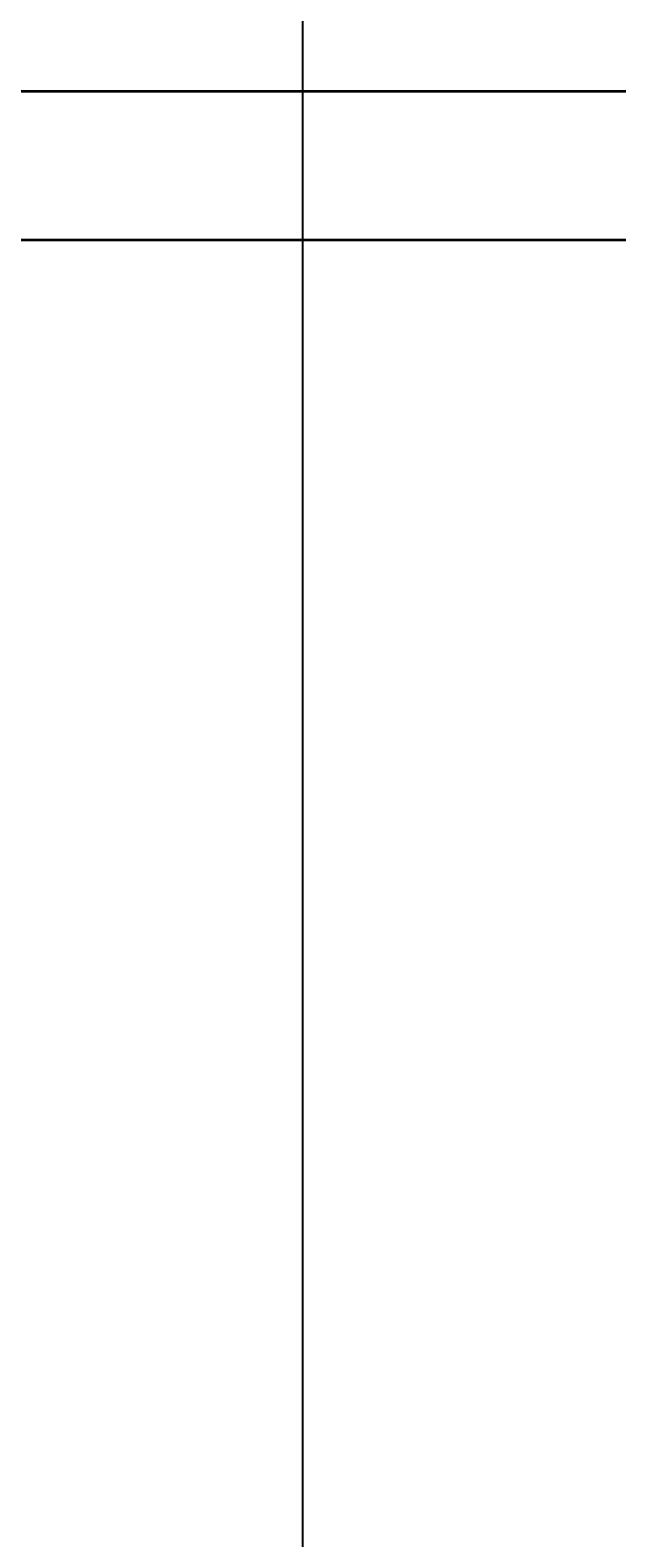
# Model space of a CAD drawing. Units: inches. Extents: x 1088 to 1703, y 668 to 1875.
# Tile 36 of 45: x 1542 to 1560, y 1629 to 1675. Entities that reach past the tile are written whole.
import ezdxf

# ---------------------------------------------------------------- set-up
doc = ezdxf.new("R2010")
doc.units = ezdxf.units.IN
doc.layers.add('A-ANNO-DIMS', color=2, linetype='Continuous', lineweight=18)
doc.layers.add('A-WALL', color=7, linetype='Continuous', lineweight=35)
doc.styles.get("Standard").update_dxf_attribs({"font": 'arial.ttf'})
doc.dimstyles.get("Standard").update_dxf_attribs({"dimtxt": 0.18, "dimasz": 0.18, "dimexe": 0.18, "dimexo": 0.0625, "dimgap": 0.09, "dimtad": 0, "dimtih": 1, "dimtoh": 1, "dimdec": 4, "dimzin": 0, "dimdsep": 46, "dimtxsty": 'Standard', "dimcen": 0.09, "dimadec": 0, "dimazin": 0, "dimtfac": 1, "dimtdec": 4, "dimtofl": 0, "dimtmove": 0, "dimatfit": 3, "dimfxl": 1, "dimtolj": 1, "dimtzin": 0, "dimarcsym": 0})

# ---------------------------------------------------------------- blocks, each defined once
blk = doc.blocks.new('*D32')
at = {"layer": 'A-ANNO-DIMS', "color": 0, "lineweight": -2, "transparency": 16777216}
for p, q in [((1550.595, 1373.121), (1550.595, 1857.788)), ((1550.775, 1857.608), (1567.825, 1857.608)), ((1585.665, 1857.608), (1568.614, 1857.608)), ((1585.845, 1360.983), (1585.845, 1857.788))]:
    blk.add_line(p, q, dxfattribs=at)
at = {"layer": 'A-ANNO-DIMS', "color": 0, "transparency": 16777216}
for points in [[(1550.775, 1857.638), (1550.775, 1857.578), (1550.595, 1857.608)], [(1585.665, 1857.638), (1585.665, 1857.578), (1585.845, 1857.608)]]:
    blk.add_solid(points, dxfattribs=at)
at = {"layer": 'Defpoints', "color": 0, "transparency": 16777216}
for p in [(1585.845, 1857.608), (1550.595, 1373.058), (1585.845, 1360.921)]:
    blk.add_point(p, dxfattribs=at)
at = {"layer": 'A-ANNO-DIMS', "color": 0, "transparency": 16777216, "insert": (1568.22, 1857.608), "char_height": 0.18, "attachment_point": 5}
blk.add_mtext('\\A1;35.25', dxfattribs=at)

msp = doc.modelspace()

# ---------------------------------------------------------------- linework, layer by layer
at = {"layer": 'A-WALL'}
for p, q in [((1481.681, 1673.058), (1585.845, 1673.058)), ((1489.845, 1668.558), (1585.845, 1668.558))]:
    msp.add_line(p, q, dxfattribs=at)

# ---------------------------------------------------------------- dimensions: what is measured, and where the dimension line sits
at = {"layer": 'A-ANNO-DIMS'}
dim = msp.add_linear_dim(base=(1585.845, 1857.608), p1=(1550.595, 1373.058), p2=(1585.845, 1360.921), dimstyle='Standard', override={"dimdec": 2, "dimlfac": 1, "dimrnd": 0, "dimzin": 0, "dimdsep": 46, "dimlunit": 2}, dxfattribs=at)
dim.commit()
dim.dimension.update_dxf_attribs({"geometry": '*D32', "text_midpoint": (1568.22, 1857.608)})

doc.saveas('drawing.dxf')
